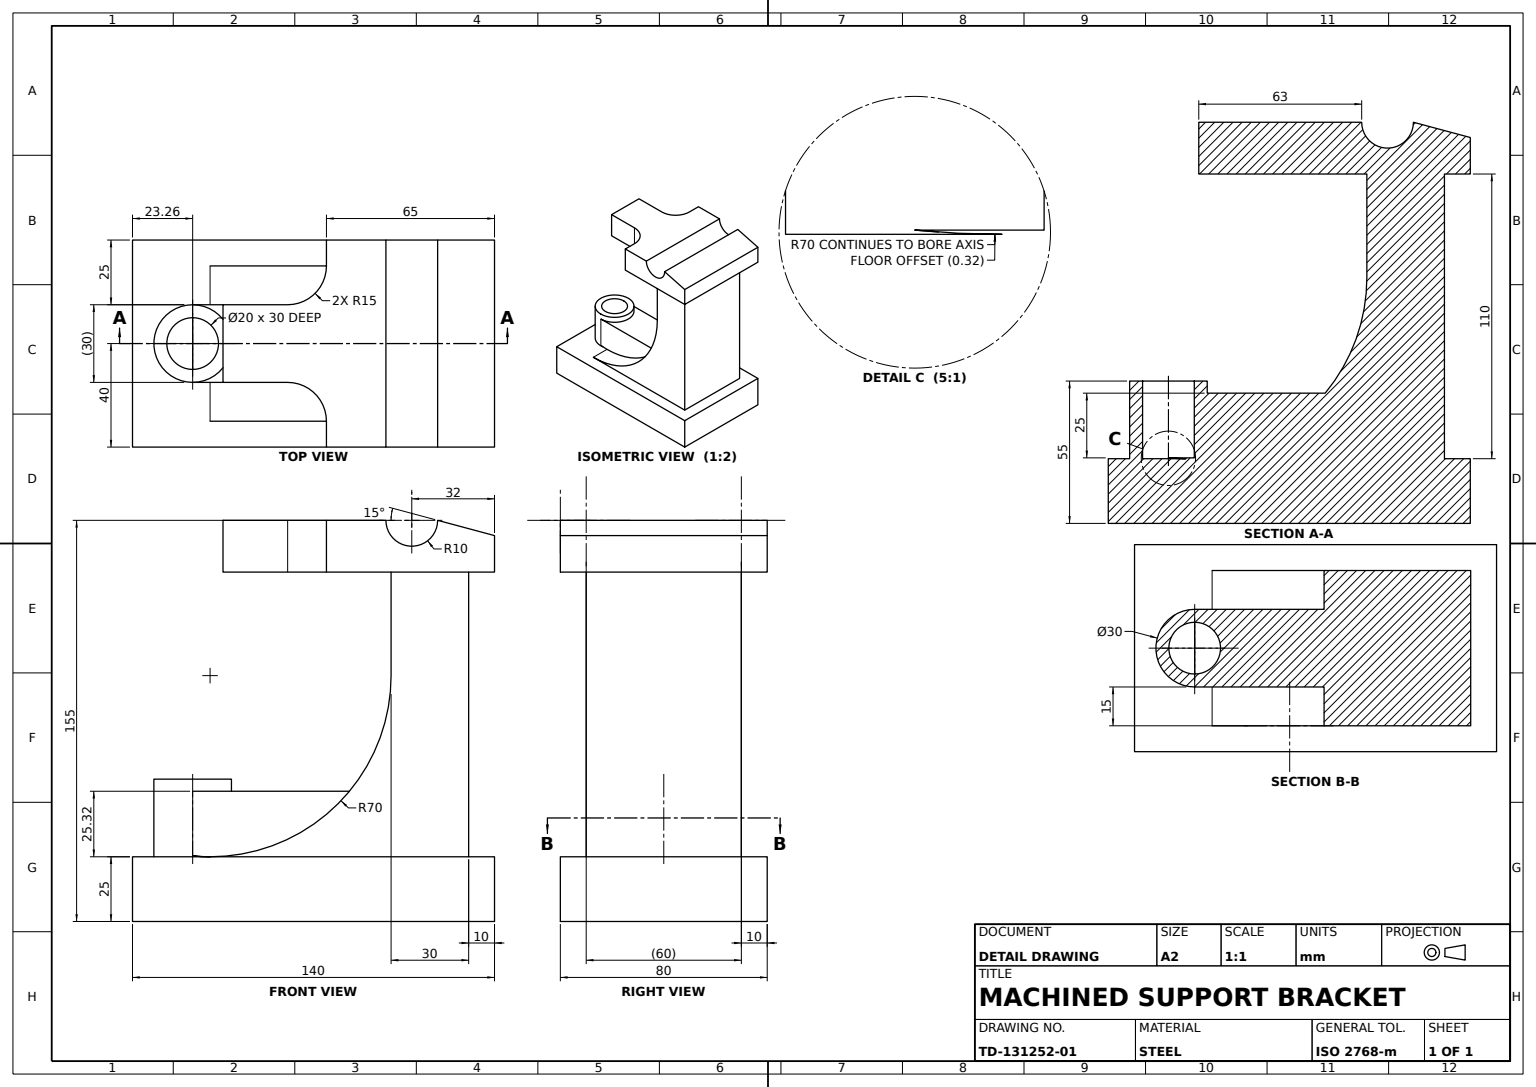
SolidWorks part; units mm, degrees
material "Plain Carbon Steel"
ref_plane "Front Plane" through (0, 0, 0) normal (0, 0, 1) x (1, 0, 0)
ref_plane "Top Plane" through (0, 0, 0) normal (0, 1, 0) x (1, 0, 0)
ref_plane "Right Plane" through (0, 0, 0) normal (1, 0, 0) x (0, 0, -1)
sketch "Bracket Profile Sketch" plane through (0, 0, 0) normal (0, 0, 1) x (1, 0, 0)
  line L0 (0, 0) -> (70, 0)
  line L1 (70, 0) -> (70, 25)
  line L2 (70, 25) -> (-70, 25)
  line L3 (-70, 25) -> (-70, 0)
  line L4 (-70, 0) -> (0, 0)
  line L5 (70, 25) -> (60, 25) construction
  line L6 (60, 25) -> (60, 135)
  line L7 (-35, 135) -> (30, 135)
  line L8 (-35, 135) -> (-35, 155)
  line L9 (-35, 155) -> (28, 155)
  line L10 (48, 155) -> (70, 155)
  line L11 (70, 155) -> (70, 135)
  line L12 (70, 135) -> (60, 135)
  line L13 (30, 135) -> (30, 95)
  arc A0 (28, 155) -> (48, 155) centre (38, 155) ccw
  arc A1 (-40, 25) -> (30, 95) centre (-40, 95) ccw
  dimension "D1" = 70
  dimension "D3" = 70
  dimension "D6" = 10
  dimension "D2" = 25
  dimension "D4" = 110
  dimension "D5" = 20
  dimension "D7" = 10
  dimension "D8" = 98.4073
  dimension "D9" = 10
  dimension "D10" = 63
  dimension "D11" = 155
  dimension "D12" = 70
  dimension "D13" = 32
extrude "Bracket Body" add sketch "Bracket Profile Sketch" along normal mid plane 80 contours A1 L2 L6 L12 L11 L10 A0 L9 L8 L7 L13 | L3 L4 L0 L1 L2
sketch "Base Recess Sketch" plane through (60, 0, 0) normal (1, 0, 0) x (0, 0, -1)
  line L0 (0, 25) -> (0, 135) construction
  line L1 (-40, 25) -> (40, 25) construction
  line L2 (-40, 135) -> (40, 135) construction
  line L4 (-40, 25) -> (40, 25) construction
  line L5 (30, 25) -> (30, 135)
  line L6 (-40, 135) -> (40, 135) construction
  line L10 (-30, 25) -> (-30, 135)
  line L13 (-30, 25) -> (0, 25)
  line L14 (-30, 25) -> (0, 25)
  line L15 (-30, 135) -> (-40, 135)
  line L16 (-40, 135) -> (-40, 25)
  line L17 (-40, 25) -> (-30, 25)
  line L18 (30, 135) -> (40, 135)
  line L19 (40, 135) -> (40, 25)
  line L20 (40, 25) -> (30, 25)
  line M8 (40, 25) -> (40, 135)
  line M9 (40, 135) -> (-40, 135)
  line M10 (-40, 135) -> (-40, 25)
  line M11 (-40, 25) -> (40, 25)
  dimension "D1" = 10
extrude "Base Recess Cut" cut sketch "Base Recess Sketch" against normal through all contours L5 M11 M8 M9 | L10 M11 M9 M10
sketch "Cradle Groove Sketch" plane through (0, 155, 0) normal (0, 1, 0) x (1, 0, 0)
  line L0 (-35, -15) -> (-35, 15)
  line L1 (-35, -40) -> (-35, 40) construction
  line L2 (-35, 15) -> (-10, 15)
  line L3 (-35, 0) -> (0, 0) construction
  line L4 (5, 30) -> (5, 40)
  line L5 (-35, 40) -> (28, 40) construction
  line L6 (5, -30) -> (5, -40)
  line L7 (-35, -15) -> (-10, -15)
  line L8 (-35, 15) -> (-35, 40)
  line L9 (-35, 40) -> (5, 40)
  line L10 (-35, -15) -> (-35, -40)
  line L11 (-35, -40) -> (5, -40)
  arc A0 (-10, 15) -> (5, 30) centre (-10, 30) ccw
  arc A1 (-10, -15) -> (5, -30) centre (-10, -30) cw
  line M12 (28, 40) -> (-35, 40)
  line M13 (-35, 40) -> (-35, -40)
  line M14 (-35, -40) -> (28, -40)
  dimension "D1" = 30
  dimension "D2" = 15
  dimension "D3" = 39.0512
extrude "Cradle Groove R15" cut sketch "Cradle Groove Sketch" against normal blind 80 contours L2 A0 L4 M12 M13 | A1 L7 L6 M13 M14
sketch "Top Chamfer Sketch" plane through (0, 0, 40) normal (0, 0, 1) x (1, 0, 0)
  line L0 (48, 155) -> (70, 149.1051)
  line L1 (48, 155) -> (70, 155)
  line L2 (70, 155) -> (70, 149.1051)
  line L3 (70, 155) -> (70, 135) construction
  dimension "D1" = 15
extrude "Top Chamfer Cut 15deg" cut sketch "Top Chamfer Sketch" against normal blind 80
sketch "Pin Boss Sketch" plane through (0, 0, 0) normal (0, 1, 0) x (1, 0, 0)
  line L0 (14.2648, 0) -> (-46.7352, 0) construction
  circle A1 centre (-46.7352, 0) radius 15
  circle A2 centre (-46.7352, 0) radius 10
  dimension "D1" = 61
  dimension "D2" = 20
  dimension "D3" = 30
  dimension "D4" = 46.7352
extrude "Pin Boss" add sketch "Pin Boss Sketch" along normal blind 55
sketch "Curved Web Sketch" plane through (0, 0, 0) normal (0, 0, 1) x (1, 0, 0)
  line L2 (-46.7352, 25.3248) -> (-46.7352, 50.3248)
  line L6 (-46.7352, 50.3248) -> (13.8899, 50.3248)
  arc A3 (-46.7352, 25.3248) -> (13.8899, 50.3248) centre (-40, 95) ccw
  dimension "D1" = 70
  dimension "D2" = 95
  dimension "D3" = 25
  dimension "D4" = 60.6251
  dimension "D5" = 40
extrude "Curved Web" add sketch "Curved Web Sketch" along normal mid plane 30
sketch "Pin Bore Sketch" plane through (0, 50.3248, 0) normal (0, 1, 0) x (1, 0, 0)
  circle A0 centre (-46.7352, 0) radius 10
  dimension "D1" = 20
extrude "Pin Bore Ø20" cut sketch "Pin Bore Sketch" against normal blind 25
